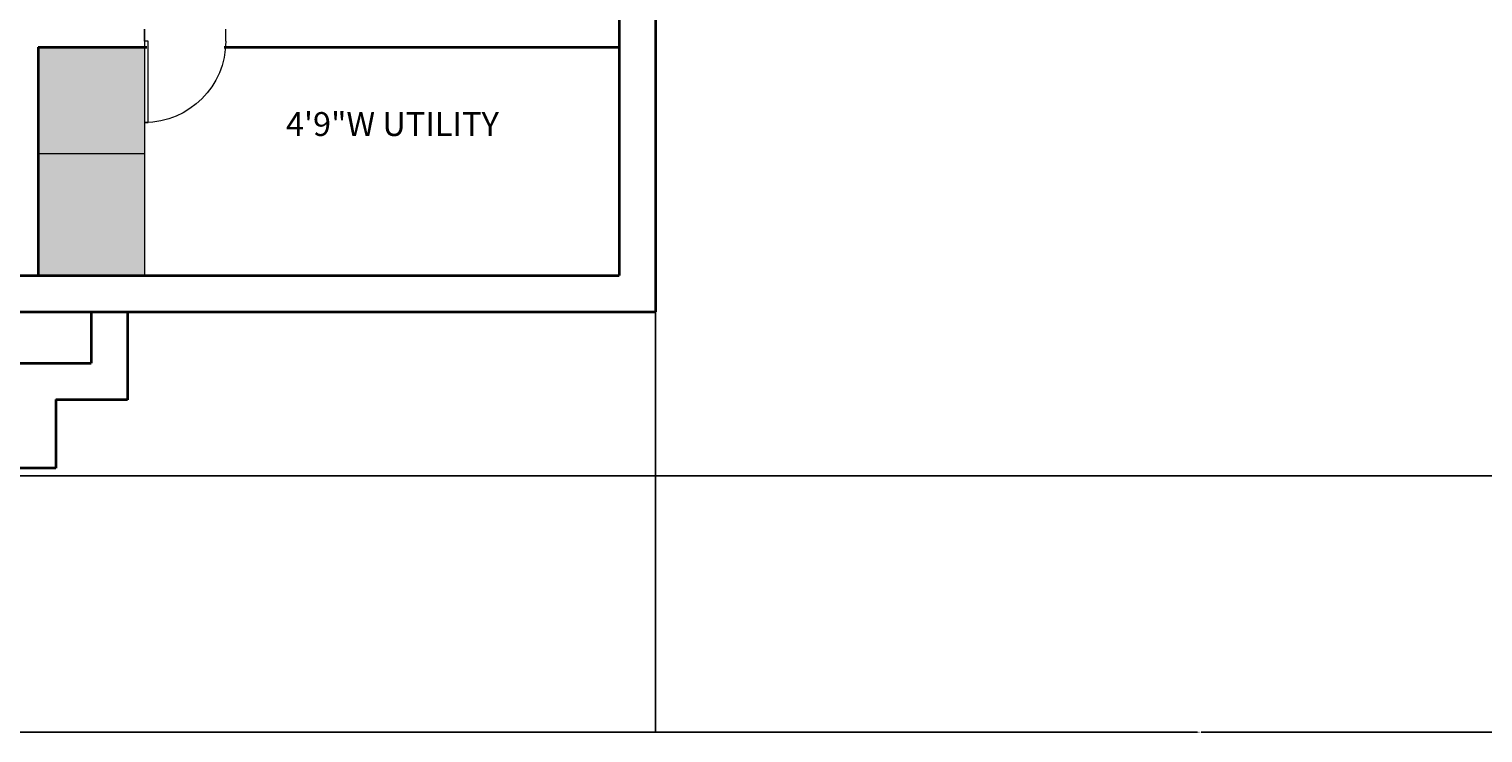
# Model space of a CAD drawing. Units: millimetres. Extents: x 27017497 to 27018854, y 7058029 to 7059154.
# Tile 48 of 91: x 27017886 to 27018246, y 7058029 to 7058203. Entities that reach past the tile are written whole.
import ezdxf

# ---------------------------------------------------------------- set-up
doc = ezdxf.new("R2010")
doc.units = ezdxf.units.MM
for name, color, linetype, lineweight in [('A-ANNO-DIMS', 2, 'Continuous', 18), ('A-AREA-IDEN', 7, 'Continuous', 18), ('A-DOOR', 4, 'Continuous', 20), ('A-FLOR-CASE', 8, 'Continuous', 20), ('A-FLOR-CASE-PATT', 44, 'Continuous', 13), ('A-WALL', 7, 'Continuous', 35)]:
    doc.layers.add(name, color=color, linetype=linetype, lineweight=lineweight)
doc.styles.get("Standard").update_dxf_attribs({"font": 'arial.ttf'})
doc.dimstyles.get("Standard").update_dxf_attribs({"dimtxt": 0.18, "dimasz": 0.18, "dimexe": 0.18, "dimexo": 0.0625, "dimgap": 0.09, "dimtad": 0, "dimtih": 1, "dimtoh": 1, "dimdec": 4, "dimzin": 0, "dimdsep": 46, "dimtxsty": 'Standard', "dimcen": 0.09, "dimadec": 0, "dimazin": 0, "dimtfac": 1, "dimtdec": 4, "dimtofl": 0, "dimtmove": 0, "dimatfit": 3, "dimfxl": 1, "dimtolj": 1, "dimtzin": 0, "dimarcsym": 0})

# ---------------------------------------------------------------- blocks, each defined once
blk = doc.blocks.new('*U2')
for p, q in [((0, 0), (0, -6)), ((40, 0), (40, -6))]:
    blk.add_line(p, q)
blk.add_lwpolyline([(0, 0), (0, 40), (1.75, 40), (1.75, 0)], close=True)
blk.add_arc((0, 0), 40, 0, 90)
blk = doc.blocks.new('*D47')
at = {"layer": 'A-ANNO-DIMS', "color": 0, "lineweight": -2, "transparency": 16777216}
for p, q in [((27017561.17, 7058294.35), (27017561.17, 7058028.6)), ((27018790.61, 7058294.35), (27018790.61, 7058028.6)), ((27017561.35, 7058028.78), (27018175.43, 7058028.78)), ((27018790.43, 7058028.78), (27018176.34, 7058028.78))]:
    blk.add_line(p, q, dxfattribs=at)
at = {"layer": 'A-ANNO-DIMS', "color": 0, "transparency": 16777216}
for points in [[(27017561.35, 7058028.81), (27017561.35, 7058028.75), (27017561.17, 7058028.78)], [(27018790.43, 7058028.81), (27018790.43, 7058028.75), (27018790.61, 7058028.78)]]:
    blk.add_solid(points, dxfattribs=at)
at = {"layer": 'Defpoints', "color": 0, "transparency": 16777216}
for p in [(27017561.17, 7058294.41), (27018790.61, 7058294.41), (27018790.61, 7058028.78)]:
    blk.add_point(p, dxfattribs=at)
at = {"layer": 'A-ANNO-DIMS', "color": 0, "transparency": 16777216, "insert": (27018175.89, 7058028.78), "char_height": 0.18, "attachment_point": 5}
blk.add_mtext('\\A1;1229.4', dxfattribs=at)
blk = doc.blocks.new('*D48')
at = {"layer": 'A-ANNO-DIMS', "color": 0, "lineweight": -2, "transparency": 16777216}
for p, q in [((27018463.5, 7058622.91), (27017497.54, 7058622.91)), ((27017497.72, 7058622.73), (27017497.72, 7058357.75)), ((27017497.72, 7058092.41), (27017497.72, 7058357.39)), ((27018555.13, 7058092.23), (27017497.54, 7058092.23))]:
    blk.add_line(p, q, dxfattribs=at)
at = {"layer": 'A-ANNO-DIMS', "color": 0, "transparency": 16777216}
for points in [[(27017497.69, 7058622.73), (27017497.75, 7058622.73), (27017497.72, 7058622.91)], [(27017497.69, 7058092.41), (27017497.75, 7058092.41), (27017497.72, 7058092.23)]]:
    blk.add_solid(points, dxfattribs=at)
at = {"layer": 'Defpoints', "color": 0, "transparency": 16777216}
for p in [(27018463.56, 7058622.91), (27017497.72, 7058092.23), (27018555.19, 7058092.23)]:
    blk.add_point(p, dxfattribs=at)
at = {"layer": 'A-ANNO-DIMS', "color": 0, "transparency": 16777216, "insert": (27017497.72, 7058357.57), "char_height": 0.18, "attachment_point": 5}
blk.add_mtext('\\A1;530.7', dxfattribs=at)
blk = doc.blocks.new('*D51')
at = {"layer": 'A-ANNO-DIMS', "color": 0, "lineweight": -2, "transparency": 16777216}
for p, q in [((27018041.17, 7058345.35), (27018041.17, 7058028.6)), ((27018310.61, 7058345.35), (27018310.61, 7058028.6)), ((27018041.35, 7058028.78), (27018175.42, 7058028.78)), ((27018310.43, 7058028.78), (27018176.35, 7058028.78))]:
    blk.add_line(p, q, dxfattribs=at)
at = {"layer": 'A-ANNO-DIMS', "color": 0, "transparency": 16777216}
for points in [[(27018041.35, 7058028.81), (27018041.35, 7058028.75), (27018041.17, 7058028.78)], [(27018310.43, 7058028.81), (27018310.43, 7058028.75), (27018310.61, 7058028.78)]]:
    blk.add_solid(points, dxfattribs=at)
at = {"layer": 'Defpoints', "color": 0, "transparency": 16777216}
for p in [(27018041.17, 7058345.41), (27018310.61, 7058345.41), (27018310.61, 7058028.78)]:
    blk.add_point(p, dxfattribs=at)
at = {"layer": 'A-ANNO-DIMS', "color": 0, "transparency": 16777216, "insert": (27018175.89, 7058028.78), "char_height": 0.18, "attachment_point": 5}
blk.add_mtext('\\A1;269.44', dxfattribs=at)

msp = doc.modelspace()

# ---------------------------------------------------------------- hatches: boundary and pattern name
at = {"layer": 'A-FLOR-CASE-PATT'}
h = msp.add_hatch(color=256, dxfattribs=at)
h.dxf.hatch_style = 1
h.paths.add_polyline_path([(27017914.521, 7058198.412), (27017888.166, 7058198.412), (27017888.166, 7058172.104), (27017914.521, 7058172.104)])
h.paths.add_polyline_path([(27017914.521, 7058172.104), (27017888.166, 7058172.104), (27017888.166, 7058141.912), (27017914.521, 7058141.912)])

# ---------------------------------------------------------------- linework, layer by layer
at = {"layer": 'A-FLOR-CASE'}
for p, q in [((27017914.521, 7058202.91), (27017914.521, 7058141.912)), ((27017888.166, 7058172.104), (27017914.521, 7058172.104))]:
    msp.add_line(p, q, dxfattribs=at)
at = {"layer": 'A-WALL'}
for p, q in [((27018032.166, 7058386.803), (27018032.166, 7058141.912)), ((27018041.166, 7058386.357), (27018041.166, 7058132.912)), ((27017888.166, 7058198.412), (27017888.166, 7058141.912)), ((27017888.166, 7058198.412), (27017915.061, 7058198.412)), ((27017934.269, 7058198.412), (27018032.166, 7058198.412)), ((27017883.666, 7058141.912), (27018032.166, 7058141.912)), ((27017883.666, 7058132.912), (27018041.166, 7058132.912)), ((27017901.33, 7058132.912), (27017901.33, 7058120.17)), ((27017910.33, 7058132.912), (27017910.33, 7058122.863)), ((27017910.332, 7058122.868), (27017910.332, 7058111.05)), ((27017883.582, 7058120.17), (27017901.33, 7058120.17)), ((27017892.582, 7058111.17), (27017892.582, 7058094.141)), ((27017892.582, 7058111.17), (27017910.332, 7058111.17)), ((27017892.582, 7058094.141), (27017802.166, 7058094.141))]:
    msp.add_line(p, q, dxfattribs=at)

# ---------------------------------------------------------------- block references
at = {"layer": 'A-DOOR', "xscale": -0.503175151877956, "yscale": 0.503175151877956, "zscale": 0.503175151877956, "rotation": 180}
msp.add_blockref('*U2', (27017914.524, 7058199.894), dxfattribs=at)

# ---------------------------------------------------------------- texts
at = {"layer": 'A-AREA-IDEN'}
msp.add_text('4\'9"W UTILITY', height=5.91176, dxfattribs=at).set_placement((27017949.55, 7058176.439))

# ---------------------------------------------------------------- dimensions: what is measured, and where the dimension line sits
at = {"layer": 'A-ANNO-DIMS'}
dim = msp.add_linear_dim(base=(27017497.716, 7058092.23), p1=(27018463.561, 7058622.912), p2=(27018555.192, 7058092.23), angle=90, dimstyle='Standard', override={"dimdec": 1, "dimlfac": 1, "dimrnd": 0, "dimzin": 0, "dimdsep": 46, "dimlunit": 2}, dxfattribs=at)
dim.commit()
dim.dimension.update_dxf_attribs({"geometry": '*D48', "text_midpoint": (27017497.716, 7058357.571)})
for base, p1, p2, override, picture in [((27018310.606, 7058028.78), (27018041.166, 7058345.412), (27018310.606, 7058345.412), {"dimdec": 2, "dimlfac": 1, "dimrnd": 0, "dimzin": 0, "dimdsep": 46, "dimlunit": 2}, '*D51'), ((27018790.606, 7058028.78), (27017561.166, 7058294.412), (27018790.606, 7058294.412), {"dimdec": 1, "dimlfac": 1, "dimrnd": 0, "dimzin": 0, "dimdsep": 46, "dimlunit": 2}, '*D47')]:
    dim = msp.add_linear_dim(base=base, p1=p1, p2=p2, dimstyle='Standard', override=override, dxfattribs=at)
    dim.commit()
    dim.dimension.update_dxf_attribs({"geometry": picture, "text_midpoint": (27018175.886, 7058028.78)})

doc.saveas('drawing.dxf')
